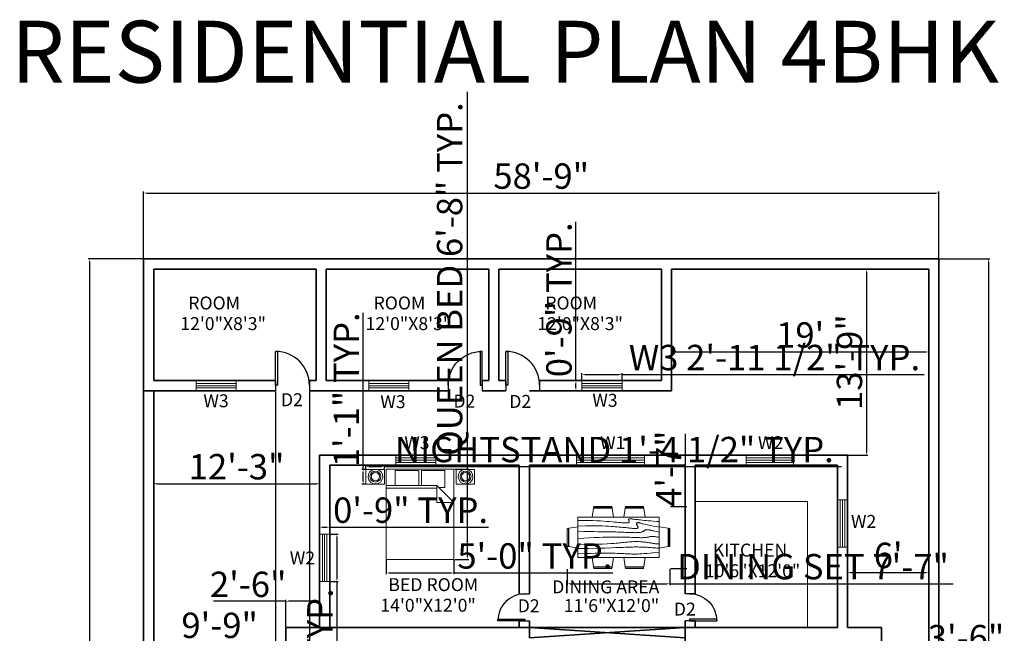
# Model space of a CAD drawing. Units: inches. Extents: x 164 to 1038, y 98 to 1358.
# Tile 4 of 4: x 164 to 1037, y 814 to 1358. Entities that reach past the tile are written whole.
import ezdxf

# ---------------------------------------------------------------- set-up
doc = ezdxf.new("R2010")
doc.units = ezdxf.units.IN
for name, color, linetype, lineweight in [('A-ANNO-DIMS', 7, 'Continuous', 18), ('A-ANNO-TEXT', 3, 'Continuous', 18), ('A-ANNO-TITL', 7, 'Continuous', 35), ('A-AREA-IDEN', 3, 'Continuous', 18), ('A-FLOR-FIXT', 2, 'Continuous', 18), ('C-SITE-WALL', 7, 'Continuous', 35), ('door', 6, 'Continuous', 25), ('furniture', 2, 'Continuous', 18), ('wall', 7, 'Continuous', 35), ('window', 10, 'Continuous', 18)]:
    doc.layers.add(name, color=color, linetype=linetype, lineweight=lineweight)
doc.styles.get("Standard").update_dxf_attribs({"font": 'arial.ttf'})
doc.dimstyles.new('ISO-25', dxfattribs={"dimtxt": 22.5, "dimasz": 2.5, "dimexe": 1.25, "dimexo": 0.625, "dimtad": 1, "dimdec": 0, "dimlunit": 3, "dimtxsty": 'Standard', "dimcen": 2.5, "dimadec": 0, "dimazin": 0, "dimtfac": 1, "dimtdec": 0, "dimtmove": 0, "dimatfit": 3, "dimfxl": 1, "dimarcsym": 0})

# ---------------------------------------------------------------- blocks, each defined once
blk = doc.blocks.new('*U3')
for p, q in [((0, 0), (0, -5)), ((30, 0), (30, -5))]:
    blk.add_line(p, q)
blk.add_lwpolyline([(0, 0), (0, 30), (1.75, 30), (1.75, 0)], close=True)
blk.add_arc((0, 0), 30, 0, 90)
blk = doc.blocks.new('Dining Set - 36 x 72 in.')
for p, q in [((-22, 27.5), (-22.1562, 26.50042)), ((-5.8416, 26.5), (-22.1534, 26.5)), ((-22, 27.5), (-6, 27.5)), ((-5.8437, 26.49966), (-6, 27.5)), ((6, 27.5), (5.8438, 26.50042)), ((22.1584, 26.5), (5.8466, 26.5)), ((6, 27.5), (22, 27.5)), ((22.1563, 26.49966), (22, 27.5)), ((36, 18), (-36, 18)), ((-36, 18), (-36, -18)), ((-22.2343, 26.00059), (-23.4847, 17.99762)), ((-22.2304, 26), (-5.7608, 26)), ((-4.5152, 17.99762), (-5.7655, 25.99926)), ((5.7657, 26.00059), (4.5153, 17.99762)), ((5.7696, 26), (22.2392, 26)), ((23.4848, 17.99762), (22.2345, 25.99926)), ((36, -18), (36, 18)), ((-44.0006, 8.23428), (-35.9976, 9.48474)), ((44.0006, 8.23428), (35.9976, 9.48474)), ((-45.5, 8), (-44.5004, 8.15617)), ((-45.5, 8), (-45.5, -8)), ((-44.5, -8.15843), (-44.5, 8.15338)), ((-44, 8.23041), (-44, -8.23915)), ((44, 8.23041), (44, -8.23915)), ((44.5, -8.15843), (44.5, 8.15338)), ((45.5, 8), (44.5005, 8.15617)), ((45.5, 8), (45.5, -8)), ((-44.4997, -8.15631), (-45.5, -8)), ((-35.9976, -9.48476), (-43.9993, -8.2345)), ((35.9976, -9.48476), (43.9993, -8.2345)), ((44.4997, -8.15631), (45.5, -8)), ((-36, -18), (36, -18)), ((-22.2343, -26.0006), (-23.4847, -17.99762)), ((-22.2304, -26), (-5.7608, -26)), ((-4.5152, -17.99762), (-5.7655, -25.99928)), ((5.7657, -26.0006), (4.5153, -17.99762)), ((5.7696, -26), (22.2392, -26)), ((23.4848, -17.99762), (22.2345, -25.99928)), ((-22, -27.5), (-22.1562, -26.50044)), ((-5.8416, -26.5), (-22.1534, -26.5)), ((-22, -27.5), (-6, -27.5)), ((-5.8437, -26.49967), (-6, -27.5)), ((6, -27.5), (5.8438, -26.50044)), ((22.1584, -26.5), (5.8466, -26.5)), ((6, -27.5), (22, -27.5)), ((22.1563, -26.49967), (22, -27.5))]:
    blk.add_line(p, q)
for points in [[(-36, 15), (-31.1772, 14.97754), (-26.8079, 14.91406), (-22.8538, 14.81543), (-19.276, 14.6875), (-16.0362, 14.53613), (-13.0957, 14.36718), (-10.4159, 14.18652), (-7.9583, 14), (-5.6904, 13.81315), (-3.6035, 13.63021), (-1.6954, 13.45508), (0.0365, 13.29166), (1.5945, 13.14388), (2.9811, 13.01562), (4.1988, 12.9108), (5.25, 12.83333), (6.1393, 12.78613), (6.8802, 12.76823), (7.4883, 12.77767), (7.9792, 12.8125), (8.3685, 12.87077), (8.6719, 12.95052), (8.9049, 13.0498), (9.0833, 13.16666), (9.2205, 13.29899), (9.3216, 13.44401), (9.3895, 13.59879), (9.4271, 13.76041), (9.4373, 13.92594), (9.4232, 14.09245), (9.3875, 14.257), (9.3333, 14.41666), (9.2638, 14.56917), (9.1836, 14.71484), (9.0975, 14.85465), (9.0104, 14.98958), (8.9272, 15.1206), (8.8529, 15.2487), (8.7922, 15.37483), (8.75, 15.5), (8.7305, 15.62467), (8.7344, 15.74739), (8.7617, 15.86621), (8.8125, 15.97916), (8.8867, 16.08431), (8.9844, 16.17968), (9.1055, 16.26334), (9.25, 16.33333), (9.4189, 16.38802), (9.6172, 16.42708), (9.8506, 16.45052), (10.125, 16.45833), (10.4463, 16.45052), (10.8203, 16.42708), (11.2529, 16.38802), (11.75, 16.33333), (12.3184, 16.26318), (12.9694, 16.17838), (13.7151, 16.07991), (14.5677, 15.96875), (15.5395, 15.84586), (16.6426, 15.71224), (17.8893, 15.56884), (19.2917, 15.41666), (20.859, 15.25667), (22.5879, 15.08984), (24.4721, 14.91715), (26.5052, 14.73958), (28.6809, 14.5581), (30.9929, 14.3737), (33.4347, 14.18733), (36, 14)], [(-36, 10), (-28.9766, 10.14274), (-23.1725, 10.20442), (-18.4241, 10.19775), (-14.5677, 10.13541), (-11.4399, 10.03011), (-8.877, 9.89453), (-6.7154, 9.74137), (-4.7917, 9.58333), (-2.9698, 9.43082), (-1.2246, 9.28515), (0.4415, 9.14534), (2.026, 9.01041), (3.5266, 8.87939), (4.9408, 8.7513), (6.266, 8.62516), (7.5, 8.5), (8.6411, 8.37549), (9.6914, 8.2539), (10.6538, 8.13818), (11.5312, 8.03125), (12.3267, 7.93603), (13.043, 7.85547), (13.6831, 7.79248), (14.25, 7.75), (14.7471, 7.7303), (15.1797, 7.73307), (15.5537, 7.75732), (15.875, 7.80208), (16.1494, 7.86637), (16.3828, 7.94922), (16.5811, 8.04964), (16.75, 8.16666), (16.8944, 8.29915), (17.0143, 8.44531), (17.1089, 8.60319), (17.1771, 8.77083), (17.218, 8.94629), (17.2305, 9.1276), (17.2137, 9.31282), (17.1667, 9.5), (17.0895, 9.6875), (16.987, 9.875), (16.8649, 10.0625), (16.7292, 10.25), (16.5856, 10.4375), (16.4401, 10.625), (16.2985, 10.8125), (16.1667, 11), (16.05, 11.18733), (15.9518, 11.3737), (15.8752, 11.5581), (15.8229, 11.73958), (15.798, 11.91715), (15.8034, 12.08984), (15.842, 12.25667), (15.9167, 12.41666), (16.0295, 12.56836), (16.1784, 12.70833), (16.3605, 12.83268), (16.5729, 12.9375), (16.8127, 13.01888), (17.0768, 13.07291), (17.3625, 13.0957), (17.6667, 13.08333), (17.9894, 13.03312), (18.3418, 12.94726), (18.7382, 12.82918), (19.1927, 12.68229), (19.7195, 12.51001), (20.3327, 12.31575), (21.0465, 12.10294), (21.875, 11.875), (22.8357, 11.63354), (23.959, 11.37304), (25.2786, 11.08618), (26.8282, 10.76562), (28.6414, 10.40405), (30.752, 9.99414), (33.1936, 9.52856), (36, 9)], [(-36, 5.5), (-30.7157, 5.3348), (-26.069, 5.20963), (-21.9946, 5.11767), (-18.4271, 5.05208), (-15.3009, 5.00602), (-12.5508, 4.97265), (-10.1112, 4.94515), (-7.9167, 4.91666), (-5.909, 4.88167), (-4.0586, 4.83984), (-2.3429, 4.79215), (-0.7396, 4.73958), (0.7739, 4.6831), (2.22, 4.6237), (3.6213, 4.56233), (5, 4.5), (6.373, 4.43782), (7.7344, 4.3776), (9.0723, 4.32129), (10.375, 4.27083), (11.6309, 4.22819), (12.8281, 4.19531), (13.9551, 4.17415), (15, 4.16666), (15.954, 4.17448), (16.819, 4.19791), (17.6001, 4.23698), (18.3021, 4.29166), (18.9299, 4.36198), (19.4883, 4.44791), (19.9823, 4.54948), (20.4167, 4.66666), (20.7969, 4.79899), (21.1302, 4.94401), (21.4245, 5.09879), (21.6875, 5.26041), (21.9271, 5.42594), (22.1511, 5.59245), (22.3672, 5.757), (22.5834, 5.91666), (22.8065, 6.06868), (23.0404, 6.21093), (23.2879, 6.34147), (23.5521, 6.45833), (23.8358, 6.55957), (24.142, 6.64323), (24.4735, 6.70735), (24.8334, 6.75), (25.2235, 6.76969), (25.642, 6.76692), (26.0858, 6.74267), (26.5521, 6.69791), (27.0379, 6.63362), (27.5404, 6.55078), (28.0565, 6.45036), (28.5834, 6.33333), (29.1242, 6.19987), (29.7071, 6.04687), (30.3661, 5.87044), (31.1354, 5.66666), (32.0493, 5.43164), (33.142, 5.16146), (34.4475, 4.85221), (36, 4.5)], [(-36, -1), (-30.7915, -0.6591), (-26.0195, -0.38216), (-21.6519, -0.16284), (-17.6563, 0.00521), (-14.0005, 0.12833), (-10.6523, 0.21289), (-7.5796, 0.26522), (-4.75, 0.29166), (-2.134, 0.29793), (0.2878, 0.28711), (2.5317, 0.26163), (4.6146, 0.22396), (6.5529, 0.17651), (8.3633, 0.12174), (10.0623, 0.06209), (11.6667, 0), (13.1899, -0.06201), (14.6341, -0.1211), (15.9982, -0.17432), (17.2813, -0.21875), (18.4823, -0.25147), (19.6003, -0.26953), (20.6343, -0.27002), (21.5834, -0.25), (22.4481, -0.20768), (23.2357, -0.14584), (23.9549, -0.06836), (24.6146, 0.02083), (25.2235, 0.11784), (25.7904, 0.21875), (26.3241, 0.31966), (26.8334, 0.41666), (27.3265, 0.50618), (27.8099, 0.58593), (28.2894, 0.65397), (28.7709, 0.70833), (29.2601, 0.74707), (29.763, 0.76823), (30.2855, 0.76985), (30.8334, 0.75), (31.4088, 0.70784), (31.9994, 0.64713), (32.589, 0.57275), (33.1615, 0.48958), (33.7008, 0.4025), (34.1908, 0.3164), (34.6153, 0.23616), (34.9584, 0.16666), (35.2099, 0.11165), (35.3848, 0.07031), (35.504, 0.04069), (35.5886, 0.02083), (35.6594, 0.00879), (35.7377, 0.0026), (35.8442, 0.00032), (36, 0)], [(-36, -6.5), (-27.1843, -6.31267), (-20.084, -6.1263), (-14.469, -5.9419), (-10.1094, -5.76042), (-6.7752, -5.58285), (-4.2363, -5.41016), (-2.2629, -5.24333), (-0.625, -5.08334), (0.8708, -4.93099), (2.2715, -4.78646), (3.5872, -4.64974), (4.8281, -4.52084), (6.0046, -4.39974), (7.127, -4.28646), (8.2053, -4.18099), (9.25, -4.08334), (10.2705, -3.99382), (11.2734, -3.91407), (12.2647, -3.84603), (13.25, -3.79167), (14.2354, -3.75293), (15.2266, -3.73177), (16.2295, -3.73015), (17.25, -3.75), (18.2912, -3.79248), (19.3451, -3.85547), (20.4009, -3.93604), (21.4479, -4.03125), (22.4754, -4.13819), (23.4727, -4.25391), (24.4289, -4.37549), (25.3334, -4.5), (26.1785, -4.62492), (26.9694, -4.74935), (27.7145, -4.87281), (28.4219, -4.99479), (29.1, -5.11483), (29.7572, -5.23242), (30.4016, -5.34709), (31.0417, -5.45834), (31.6837, -5.56437), (32.3262, -5.65821), (32.9658, -5.73153), (33.599, -5.77604), (34.2224, -5.78345), (34.8327, -5.74545), (35.4264, -5.65373), (36, -5.5)], [(-36, -10), (-26.4022, -9.81299), (-18.4675, -9.62891), (-11.9839, -9.45069), (-6.7396, -9.28125), (-2.5226, -9.12354), (0.8789, -8.98047), (3.6769, -8.85498), (6.0833, -8.75), (8.2767, -8.66765), (10.3021, -8.60677), (12.1712, -8.56543), (13.8958, -8.54167), (15.4876, -8.53353), (16.9583, -8.53907), (18.3197, -8.55632), (19.5834, -8.58334), (20.7616, -8.61841), (21.8685, -8.66081), (22.9188, -8.71004), (23.9271, -8.76563), (24.9081, -8.82707), (25.8763, -8.89388), (26.8465, -8.96558), (27.8334, -9.04167), (28.8474, -9.12118), (29.8828, -9.20117), (30.93, -9.27824), (31.9792, -9.34896), (33.0205, -9.40991), (34.0443, -9.45768), (35.0407, -9.48885), (36, -9.5)], [(-36, -14.5), (-30.0881, -14.33513), (-25.0332, -14.21224), (-20.7312, -14.12647), (-17.0781, -14.07292), (-13.97, -14.04671), (-11.3027, -14.04297), (-8.9724, -14.05681), (-6.875, -14.08334), (-4.9224, -14.11833), (-3.0905, -14.16016), (-1.3709, -14.20785), (0.2448, -14.26042), (1.7647, -14.3169), (3.1973, -14.3763), (4.5507, -14.43767), (5.8333, -14.5), (7.0554, -14.5621), (8.235, -14.62175), (9.3922, -14.67652), (10.5469, -14.72396), (11.7192, -14.76164), (12.929, -14.78711), (14.1965, -14.79794), (15.5417, -14.79167), (16.9933, -14.76424), (18.6152, -14.70508), (20.4804, -14.60197), (22.6615, -14.44271), (25.2312, -14.21509), (28.2624, -13.9069), (31.8277, -13.50594), (36, -13)]]:
    blk.add_lwpolyline(points)
blk = doc.blocks.new('Bed - Queen')
for p, q in [((0, -80.00003), (0, 0)), ((0, 0), (59.99999, 0)), ((59.99999, 0), (59.99999, -80.00003)), ((7.99999, -1.2), (28.79998, -1.2)), ((7.99999, -14.4), (7.99999, -1.2)), ((28.79998, -1.2), (28.79998, -14.4)), ((31.19999, -1.2), (51.99999, -1.2)), ((31.19999, -14.4), (31.19999, -1.2)), ((51.99999, -1.2), (51.99999, -16.4)), ((0, -14.4), (44.8, -14.4)), ((44.8, -16.8), (0, -16.8)), ((59.99999, -29.6), (44.8, -14.4)), ((44.8, -14.4), (44.8, -29.6)), ((51.99999, -16.4), (46.79936, -16.4)), ((44.8, -29.6), (59.99999, -29.6)), ((59.99999, -80.00003), (0, -80.00003))]:
    blk.add_line(p, q)
blk = doc.blocks.new('*D17')
at = {"layer": 'A-ANNO-DIMS', "color": 0, "lineweight": -2, "transparency": 16777216}
for p, q in [((274.07, 1146.49), (274.07, 1205.54)), ((276.57, 1204.29), (976.57, 1204.29)), ((979.07, 1146.49), (979.07, 1205.54))]:
    blk.add_line(p, q, dxfattribs=at)
at = {"layer": 'A-ANNO-DIMS', "color": 0, "transparency": 16777216}
for points in [[(276.57, 1204.71), (276.57, 1203.88), (274.07, 1204.29)], [(976.57, 1204.71), (976.57, 1203.88), (979.07, 1204.29)]]:
    blk.add_solid(points, dxfattribs=at)
at = {"layer": 'Defpoints', "color": 0, "transparency": 16777216}
for p in [(979.07, 1204.29), (274.07, 1145.87), (979.07, 1145.87)]:
    blk.add_point(p, dxfattribs=at)
at = {"layer": 'A-ANNO-DIMS', "color": 0, "transparency": 16777216, "insert": (626.57, 1216.41), "char_height": 22.5, "attachment_point": 5}
blk.add_mtext('58\'-9"', dxfattribs=at)
blk = doc.blocks.new('*D19')
at = {"layer": 'A-ANNO-DIMS', "color": 0, "lineweight": -2, "transparency": 16777216}
for p, q in [((979.69, 1145.87), (1024.11, 1145.87)), ((1022.86, 1143.37), (1022.86, 212.37)), ((979.69, 209.87), (1024.11, 209.87))]:
    blk.add_line(p, q, dxfattribs=at)
at = {"layer": 'A-ANNO-DIMS', "color": 0, "transparency": 16777216}
for points in [[(1022.44, 1143.37), (1023.28, 1143.37), (1022.86, 1145.87)], [(1022.44, 212.37), (1023.28, 212.37), (1022.86, 209.87)]]:
    blk.add_solid(points, dxfattribs=at)
at = {"layer": 'Defpoints', "color": 0, "transparency": 16777216}
for p in [(979.07, 1145.87), (979.07, 209.87), (1022.86, 209.87)]:
    blk.add_point(p, dxfattribs=at)
at = {"layer": 'A-ANNO-DIMS', "color": 0, "transparency": 16777216, "insert": (1010.75, 677.87), "char_height": 22.5, "attachment_point": 5, "rotation": 90}
blk.add_mtext("78'", dxfattribs=at)
blk = doc.blocks.new('*D20')
at = {"layer": 'A-ANNO-DIMS', "color": 0, "lineweight": -2, "transparency": 16777216}
for p, q in [((273.44, 1145.87), (224.94, 1145.87)), ((226.19, 1143.37), (226.19, 212.37)), ((273.44, 209.87), (224.94, 209.87))]:
    blk.add_line(p, q, dxfattribs=at)
at = {"layer": 'A-ANNO-DIMS', "color": 0, "transparency": 16777216}
for points in [[(225.78, 1143.37), (226.61, 1143.37), (226.19, 1145.87)], [(225.78, 212.37), (226.61, 212.37), (226.19, 209.87)]]:
    blk.add_solid(points, dxfattribs=at)
at = {"layer": 'Defpoints', "color": 0, "transparency": 16777216}
for p in [(274.07, 1145.87), (226.19, 209.87), (274.07, 209.87)]:
    blk.add_point(p, dxfattribs=at)
at = {"layer": 'A-ANNO-DIMS', "color": 0, "transparency": 16777216, "insert": (214.08, 677.87), "char_height": 22.5, "attachment_point": 5, "rotation": 90}
blk.add_mtext("78'", dxfattribs=at)
blk = doc.blocks.new('*D21')
at = {"layer": 'A-ANNO-DIMS', "color": 0, "lineweight": -2, "transparency": 16777216}
for p, q in [((742.07, 1029.49), (742.07, 1064.58)), ((744.57, 1063.33), (967.57, 1063.33)), ((970.07, 1029.49), (970.07, 1064.58))]:
    blk.add_line(p, q, dxfattribs=at)
at = {"layer": 'A-ANNO-DIMS', "color": 0, "transparency": 16777216}
for points in [[(744.57, 1063.75), (744.57, 1062.92), (742.07, 1063.33)], [(967.57, 1063.75), (967.57, 1062.92), (970.07, 1063.33)]]:
    blk.add_solid(points, dxfattribs=at)
at = {"layer": 'Defpoints', "color": 0, "transparency": 16777216}
for p in [(970.07, 1063.33), (742.07, 1028.87), (970.07, 1028.87)]:
    blk.add_point(p, dxfattribs=at)
at = {"layer": 'A-ANNO-DIMS', "color": 0, "transparency": 16777216, "insert": (856.07, 1075.45), "char_height": 22.5, "attachment_point": 5}
blk.add_mtext("19'", dxfattribs=at)
blk = doc.blocks.new('*D22')
at = {"layer": 'A-ANNO-DIMS', "color": 0, "lineweight": -2, "transparency": 16777216}
for p, q in [((850.76, 1136.87), (916.03, 1136.87)), ((914.78, 1134.37), (914.78, 974.37)), ((850.76, 971.87), (916.03, 971.87))]:
    blk.add_line(p, q, dxfattribs=at)
at = {"layer": 'A-ANNO-DIMS', "color": 0, "transparency": 16777216}
for points in [[(914.36, 1134.37), (915.19, 1134.37), (914.78, 1136.87)], [(914.36, 974.37), (915.19, 974.37), (914.78, 971.87)]]:
    blk.add_solid(points, dxfattribs=at)
at = {"layer": 'Defpoints', "color": 0, "transparency": 16777216}
for p in [(850.14, 1136.87), (850.14, 971.87), (914.78, 971.87)]:
    blk.add_point(p, dxfattribs=at)
at = {"layer": 'A-ANNO-DIMS', "color": 0, "transparency": 16777216, "insert": (902.65, 1054.37), "char_height": 22.5, "attachment_point": 5, "rotation": 90}
blk.add_mtext('13\'-9"', dxfattribs=at)
blk = doc.blocks.new('*D23')
at = {"layer": 'A-ANNO-DIMS', "color": 0, "lineweight": -2, "transparency": 16777216}
for p, q in [((283.07, 908.78), (283.07, 947.73)), ((285.57, 946.48), (427.57, 946.48)), ((430.07, 908.78), (430.07, 947.73))]:
    blk.add_line(p, q, dxfattribs=at)
at = {"layer": 'A-ANNO-DIMS', "color": 0, "transparency": 16777216}
for points in [[(285.57, 946.9), (285.57, 946.06), (283.07, 946.48)], [(427.57, 946.9), (427.57, 946.06), (430.07, 946.48)]]:
    blk.add_solid(points, dxfattribs=at)
at = {"layer": 'Defpoints', "color": 0, "transparency": 16777216}
for p in [(430.07, 946.48), (283.07, 908.16), (430.07, 908.16)]:
    blk.add_point(p, dxfattribs=at)
at = {"layer": 'A-ANNO-DIMS', "color": 0, "transparency": 16777216, "insert": (356.57, 958.6), "char_height": 22.5, "attachment_point": 5}
blk.add_mtext('12\'-3"', dxfattribs=at)
blk = doc.blocks.new('*D24')
at = {"layer": 'A-ANNO-DIMS', "color": 0, "lineweight": -2, "transparency": 16777216}
for p, q in [((283.07, 795.15), (283.07, 807.04)), ((285.57, 805.79), (397.57, 805.79)), ((400.07, 795.15), (400.07, 807.04))]:
    blk.add_line(p, q, dxfattribs=at)
at = {"layer": 'A-ANNO-DIMS', "color": 0, "transparency": 16777216}
for points in [[(285.57, 806.21), (285.57, 805.37), (283.07, 805.79)], [(397.57, 806.21), (397.57, 805.37), (400.07, 805.79)]]:
    blk.add_solid(points, dxfattribs=at)
at = {"layer": 'Defpoints', "color": 0, "transparency": 16777216}
for p in [(400.07, 805.79), (283.07, 794.52), (400.07, 794.52)]:
    blk.add_point(p, dxfattribs=at)
at = {"layer": 'A-ANNO-DIMS', "color": 0, "transparency": 16777216, "insert": (341.57, 817.9), "char_height": 22.5, "attachment_point": 5}
blk.add_mtext('9\'-9"', dxfattribs=at)
blk = doc.blocks.new('*D27')
at = {"layer": 'A-ANNO-DIMS', "color": 0, "lineweight": -2, "transparency": 16777216}
for p, q in [((898.07, 871.04), (898.07, 866.59)), ((900.57, 867.84), (967.57, 867.84)), ((970.07, 871.04), (970.07, 866.59))]:
    blk.add_line(p, q, dxfattribs=at)
at = {"layer": 'A-ANNO-DIMS', "color": 0, "transparency": 16777216}
for points in [[(900.57, 868.25), (900.57, 867.42), (898.07, 867.84)], [(967.57, 868.25), (967.57, 867.42), (970.07, 867.84)]]:
    blk.add_solid(points, dxfattribs=at)
at = {"layer": 'Defpoints', "color": 0, "transparency": 16777216}
for p in [(898.07, 871.66), (970.07, 871.66), (970.07, 867.84)]:
    blk.add_point(p, dxfattribs=at)
at = {"layer": 'A-ANNO-DIMS', "color": 0, "transparency": 16777216, "insert": (934.07, 879.95), "char_height": 22.5, "attachment_point": 5}
blk.add_mtext("6'", dxfattribs=at)
blk = doc.blocks.new('*D28')
at = {"layer": 'A-ANNO-DIMS', "color": 0, "lineweight": -2, "transparency": 16777216}
for p, q in [((928.07, 772.18), (928.07, 796.13)), ((930.57, 794.88), (967.57, 794.88)), ((970.07, 772.18), (970.07, 796.13)), ((970.07, 794.88), (1033.61, 794.88))]:
    blk.add_line(p, q, dxfattribs=at)
at = {"layer": 'A-ANNO-DIMS', "color": 0, "transparency": 16777216}
for points in [[(930.57, 795.3), (930.57, 794.46), (928.07, 794.88)], [(967.57, 795.3), (967.57, 794.46), (970.07, 794.88)]]:
    blk.add_solid(points, dxfattribs=at)
at = {"layer": 'Defpoints', "color": 0, "transparency": 16777216}
for p in [(970.07, 794.88), (928.07, 771.56), (970.07, 771.56)]:
    blk.add_point(p, dxfattribs=at)
at = {"layer": 'A-ANNO-DIMS', "color": 0, "transparency": 16777216, "insert": (1003.09, 807), "char_height": 22.5, "attachment_point": 5}
blk.add_mtext('3\'-6"', dxfattribs=at)
blk = doc.blocks.new('*D29')
at = {"layer": 'A-ANNO-DIMS', "color": 0, "lineweight": -2, "transparency": 16777216}
for p, q in [((400.07, 842.17), (336.12, 842.17)), ((400.07, 819.49), (400.07, 843.42)), ((427.57, 842.17), (402.57, 842.17)), ((430.07, 819.49), (430.07, 843.42))]:
    blk.add_line(p, q, dxfattribs=at)
at = {"layer": 'A-ANNO-DIMS', "color": 0, "transparency": 16777216}
for points in [[(402.57, 842.59), (402.57, 841.75), (400.07, 842.17)], [(427.57, 842.59), (427.57, 841.75), (430.07, 842.17)]]:
    blk.add_solid(points, dxfattribs=at)
at = {"layer": 'Defpoints', "color": 0, "transparency": 16777216}
for p in [(400.07, 842.17), (400.07, 818.87), (430.07, 818.87)]:
    blk.add_point(p, dxfattribs=at)
at = {"layer": 'A-ANNO-DIMS', "color": 0, "transparency": 16777216, "insert": (366.84, 854.28), "char_height": 22.5, "attachment_point": 5}
blk.add_mtext('2\'-6"', dxfattribs=at)
blk = doc.blocks.new('WINDOW-W3')
for p, q in [((0, 9), (0, 0)), ((0, 9), (0, 0)), ((35.59, 9), (35.59, 0)), ((35.59, 9), (35.59, 0)), ((0, 6.5), (35.59, 6.5)), ((0, 6.5), (35.59, 6.5)), ((0, 4.5), (35.59, 4.5)), ((0, 4.5), (35.59, 4.5)), ((0, 2.5), (35.59, 2.5)), ((0, 2.5), (35.59, 2.5))]:
    blk.add_line(p, q)
blk = doc.blocks.new('WINDOW-W1')
for p, q in [((0, 9), (0, 0)), ((60.11, 9), (60.11, 0)), ((0, 6.5), (60.11, 6.5)), ((0, 4.5), (60.11, 4.5)), ((0, 2.5), (60.11, 2.5))]:
    blk.add_line(p, q)
blk = doc.blocks.new('WINDOW-W2')
for p, q in [((0, 9), (0, 0)), ((42.02, 9), (42.02, 0)), ((0, 6.5), (42.02, 6.5)), ((0, 4.5), (42.02, 4.5)), ((0, 2.5), (42.02, 2.5))]:
    blk.add_line(p, q)
blk = doc.blocks.new('BEDSIDE-TABLE')
blk.add_lwpolyline([(0, 13.01), (16.36, 13.01), (16.36, 0), (0, 0)], close=True)
for radius in [4.87, 3.63]:
    blk.add_circle((8.46, 6.65), radius)
blk.add_arc((8.46, 6.65), 6.51, 102.02927, 77.97073)
blk.add_arc((8.46, 6.65), 6.51, 102.02927, 77.97073)
blk = doc.blocks.new('*D36')
at = {"layer": 'A-ANNO-DIMS', "color": 0, "lineweight": -2, "transparency": 16777216}
for p, q in [((439.69, 901.66), (446.62, 901.66)), ((445.37, 899.16), (445.37, 862.14)), ((439.69, 859.64), (446.62, 859.64)), ((445.37, 859.64), (445.37, 661.94))]:
    blk.add_line(p, q, dxfattribs=at)
at = {"layer": 'A-ANNO-DIMS', "color": 0, "transparency": 16777216}
for points in [[(444.95, 899.16), (445.79, 899.16), (445.37, 901.66)], [(444.95, 862.14), (445.79, 862.14), (445.37, 859.64)]]:
    blk.add_solid(points, dxfattribs=at)
at = {"layer": 'Defpoints', "color": 0, "transparency": 16777216}
for p in [(439.07, 901.66), (439.07, 859.64), (445.37, 859.64)]:
    blk.add_point(p, dxfattribs=at)
at = {"layer": 'A-ANNO-DIMS', "color": 0, "transparency": 16777216, "insert": (433.25, 759.54), "char_height": 22.5, "attachment_point": 5, "rotation": 90}
blk.add_mtext('W2 3\'-6" TYP.', dxfattribs=at)
blk = doc.blocks.new('*D37')
at = {"layer": 'A-ANNO-DIMS', "color": 0, "lineweight": -2, "transparency": 16777216}
for p, q in [((430.07, 902.28), (430.07, 909.21)), ((432.57, 907.96), (436.57, 907.96)), ((439.07, 902.28), (439.07, 909.21)), ((439.07, 907.96), (579.97, 907.96))]:
    blk.add_line(p, q, dxfattribs=at)
at = {"layer": 'A-ANNO-DIMS', "color": 0, "transparency": 16777216}
for points in [[(432.57, 908.38), (432.57, 907.54), (430.07, 907.96)], [(436.57, 908.38), (436.57, 907.54), (439.07, 907.96)]]:
    blk.add_solid(points, dxfattribs=at)
at = {"layer": 'Defpoints', "color": 0, "transparency": 16777216}
for p in [(439.07, 907.96), (430.07, 901.66), (439.07, 901.66)]:
    blk.add_point(p, dxfattribs=at)
at = {"layer": 'A-ANNO-DIMS', "color": 0, "transparency": 16777216, "insert": (510.77, 920.07), "char_height": 22.5, "attachment_point": 5}
blk.add_mtext('0\'-9" TYP.', dxfattribs=at)
blk = doc.blocks.new('*D38')
at = {"layer": 'A-ANNO-DIMS', "color": 0, "lineweight": -2, "transparency": 16777216}
for p, q in [((662.65, 1038.49), (662.65, 1044.45)), ((665.15, 1043.2), (695.74, 1043.2)), ((698.24, 1038.49), (698.24, 1044.45)), ((698.24, 1043.2), (965.85, 1043.2))]:
    blk.add_line(p, q, dxfattribs=at)
at = {"layer": 'A-ANNO-DIMS', "color": 0, "transparency": 16777216}
for points in [[(665.15, 1043.62), (665.15, 1042.79), (662.65, 1043.2)], [(695.74, 1043.62), (695.74, 1042.79), (698.24, 1043.2)]]:
    blk.add_solid(points, dxfattribs=at)
at = {"layer": 'Defpoints', "color": 0, "transparency": 16777216}
for p in [(698.24, 1043.2), (662.65, 1037.87), (698.24, 1037.87)]:
    blk.add_point(p, dxfattribs=at)
at = {"layer": 'A-ANNO-DIMS', "color": 0, "transparency": 16777216, "insert": (833.29, 1055.47), "char_height": 22.5, "attachment_point": 5}
blk.add_mtext('W3 2\'-11 1/2" TYP.', dxfattribs=at)
blk = doc.blocks.new('*D39')
at = {"layer": 'A-ANNO-DIMS', "color": 0, "lineweight": -2, "transparency": 16777216}
for p, q in [((657.31, 1037.87), (657.31, 1178.76)), ((662.02, 1037.87), (656.06, 1037.87)), ((657.31, 1031.37), (657.31, 1035.37)), ((662.02, 1028.87), (656.06, 1028.87))]:
    blk.add_line(p, q, dxfattribs=at)
at = {"layer": 'A-ANNO-DIMS', "color": 0, "transparency": 16777216}
for points in [[(656.89, 1035.37), (657.73, 1035.37), (657.31, 1037.87)], [(656.89, 1031.37), (657.73, 1031.37), (657.31, 1028.87)]]:
    blk.add_solid(points, dxfattribs=at)
at = {"layer": 'Defpoints', "color": 0, "transparency": 16777216}
for p in [(657.31, 1037.87), (662.65, 1037.87), (662.65, 1028.87)]:
    blk.add_point(p, dxfattribs=at)
at = {"layer": 'A-ANNO-DIMS', "color": 0, "transparency": 16777216, "insert": (645.2, 1109.57), "char_height": 22.5, "attachment_point": 5, "rotation": 90}
blk.add_mtext('0\'-9" TYP.', dxfattribs=at)
blk = doc.blocks.new('*D40')
at = {"layer": 'A-ANNO-DIMS', "color": 0, "lineweight": -2, "transparency": 16777216}
for p, q in [((561.22, 959.36), (561.22, 1294.09)), ((549.84, 959.36), (562.47, 959.36)), ((561.22, 881.86), (561.22, 956.86)), ((549.84, 879.36), (562.47, 879.36))]:
    blk.add_line(p, q, dxfattribs=at)
at = {"layer": 'A-ANNO-DIMS', "color": 0, "transparency": 16777216}
for points in [[(560.8, 956.86), (561.63, 956.86), (561.22, 959.36)], [(560.8, 881.86), (561.63, 881.86), (561.22, 879.36)]]:
    blk.add_solid(points, dxfattribs=at)
at = {"layer": 'Defpoints', "color": 0, "transparency": 16777216}
for p in [(549.22, 959.36), (561.22, 959.36), (549.22, 879.36)]:
    blk.add_point(p, dxfattribs=at)
at = {"layer": 'A-ANNO-DIMS', "color": 0, "transparency": 16777216, "insert": (548.27, 1127.98), "char_height": 22.5, "attachment_point": 5, "rotation": 90}
blk.add_mtext('QUEEN BED 6\'-8" TYP.', dxfattribs=at)
blk = doc.blocks.new('*D41')
at = {"layer": 'A-ANNO-DIMS', "color": 0, "lineweight": -2, "transparency": 16777216}
for p, q in [((489.22, 878.74), (489.22, 866.11)), ((549.22, 878.74), (549.22, 866.11)), ((491.72, 867.36), (546.72, 867.36)), ((549.22, 867.36), (690.11, 867.36))]:
    blk.add_line(p, q, dxfattribs=at)
at = {"layer": 'A-ANNO-DIMS', "color": 0, "transparency": 16777216}
for points in [[(491.72, 867.78), (491.72, 866.95), (489.22, 867.36)], [(546.72, 867.78), (546.72, 866.95), (549.22, 867.36)]]:
    blk.add_solid(points, dxfattribs=at)
at = {"layer": 'Defpoints', "color": 0, "transparency": 16777216}
for p in [(489.22, 879.36), (549.22, 879.36), (549.22, 867.36)]:
    blk.add_point(p, dxfattribs=at)
at = {"layer": 'A-ANNO-DIMS', "color": 0, "transparency": 16777216, "insert": (620.92, 879.48), "char_height": 22.5, "attachment_point": 5}
blk.add_mtext('5\'-0" TYP.', dxfattribs=at)
blk = doc.blocks.new('*D42')
at = {"layer": 'A-ANNO-DIMS', "color": 0, "lineweight": -2, "transparency": 16777216}
for p, q in [((471.16, 959.77), (471.16, 962.84)), ((473.66, 961.59), (485.01, 961.59)), ((487.51, 959.77), (487.51, 962.84)), ((487.51, 961.59), (892.8, 961.59))]:
    blk.add_line(p, q, dxfattribs=at)
at = {"layer": 'A-ANNO-DIMS', "color": 0, "transparency": 16777216}
for points in [[(473.66, 962.01), (473.66, 961.18), (471.16, 961.59)], [(485.01, 962.01), (485.01, 961.18), (487.51, 961.59)]]:
    blk.add_solid(points, dxfattribs=at)
at = {"layer": 'Defpoints', "color": 0, "transparency": 16777216}
for p in [(487.51, 961.59), (471.16, 959.14), (487.51, 959.14)]:
    blk.add_point(p, dxfattribs=at)
at = {"layer": 'A-ANNO-DIMS', "color": 0, "transparency": 16777216, "insert": (691.4, 973.85), "char_height": 22.5, "attachment_point": 5}
blk.add_mtext('NIGHTSTAND 1\'-4 1/2" TYP.', dxfattribs=at)
blk = doc.blocks.new('*D43')
at = {"layer": 'A-ANNO-DIMS', "color": 0, "lineweight": -2, "transparency": 16777216}
for p, q in [((468.7, 959.14), (468.7, 1097.92)), ((470.53, 959.14), (467.45, 959.14)), ((468.7, 948.63), (468.7, 956.64)), ((470.53, 946.13), (467.45, 946.13))]:
    blk.add_line(p, q, dxfattribs=at)
at = {"layer": 'A-ANNO-DIMS', "color": 0, "transparency": 16777216}
for points in [[(468.29, 956.64), (469.12, 956.64), (468.7, 959.14)], [(468.29, 948.63), (469.12, 948.63), (468.7, 946.13)]]:
    blk.add_solid(points, dxfattribs=at)
at = {"layer": 'Defpoints', "color": 0, "transparency": 16777216}
for p in [(468.7, 959.14), (471.16, 959.14), (471.16, 946.13)]:
    blk.add_point(p, dxfattribs=at)
at = {"layer": 'A-ANNO-DIMS', "color": 0, "transparency": 16777216, "insert": (456.77, 1029.78), "char_height": 22.5, "attachment_point": 5, "rotation": 90}
blk.add_mtext('1\'-1" TYP.', dxfattribs=at)
blk = doc.blocks.new('*D48')
at = {"layer": 'A-ANNO-DIMS', "color": 0, "lineweight": -2, "transparency": 16777216}
for p, q in [((649.65, 870.75), (649.65, 856.47)), ((740.65, 870.75), (740.65, 856.47)), ((652.15, 857.72), (738.15, 857.72)), ((740.65, 857.72), (991.7, 857.72))]:
    blk.add_line(p, q, dxfattribs=at)
at = {"layer": 'A-ANNO-DIMS', "color": 0, "transparency": 16777216}
for points in [[(652.15, 858.14), (652.15, 857.31), (649.65, 857.72)], [(738.15, 858.14), (738.15, 857.31), (740.65, 857.72)]]:
    blk.add_solid(points, dxfattribs=at)
at = {"layer": 'Defpoints', "color": 0, "transparency": 16777216}
for p in [(649.65, 871.37), (740.65, 871.37), (740.65, 857.72)]:
    blk.add_point(p, dxfattribs=at)
at = {"layer": 'A-ANNO-DIMS', "color": 0, "transparency": 16777216, "insert": (867.42, 869.98), "char_height": 22.5, "attachment_point": 5}
blk.add_mtext('DINING SET 7\'-7"', dxfattribs=at)
blk = doc.blocks.new('*D49')
at = {"layer": 'A-ANNO-DIMS', "color": 0, "lineweight": -2, "transparency": 16777216}
for p, q in [((754.3, 926.37), (754.3, 990.84)), ((741.27, 926.37), (755.55, 926.37)), ((754.3, 873.87), (754.3, 923.87)), ((741.27, 871.37), (755.55, 871.37))]:
    blk.add_line(p, q, dxfattribs=at)
at = {"layer": 'A-ANNO-DIMS', "color": 0, "transparency": 16777216}
for points in [[(753.88, 923.87), (754.72, 923.87), (754.3, 926.37)], [(753.88, 873.87), (754.72, 873.87), (754.3, 871.37)]]:
    blk.add_solid(points, dxfattribs=at)
at = {"layer": 'Defpoints', "color": 0, "transparency": 16777216}
for p in [(740.65, 926.37), (754.3, 926.37), (740.65, 871.37)]:
    blk.add_point(p, dxfattribs=at)
at = {"layer": 'A-ANNO-DIMS', "color": 0, "transparency": 16777216, "insert": (742.42, 959.86), "char_height": 22.5, "attachment_point": 5, "rotation": 90}
blk.add_mtext('4\'-7"', dxfattribs=at)
blk = doc.blocks.new('*D54')
at = {"layer": 'A-ANNO-DIMS', "color": 0, "lineweight": -2, "transparency": 16777216}
for p, q in [((391.07, 1028.24), (391.07, 152.07)), ((421.07, 1028.24), (421.07, 152.07)), ((393.57, 153.32), (418.57, 153.32)), ((421.07, 153.32), (485.01, 153.32))]:
    blk.add_line(p, q, dxfattribs=at)
at = {"layer": 'A-ANNO-DIMS', "color": 0, "transparency": 16777216}
for points in [[(393.57, 153.73), (393.57, 152.9), (391.07, 153.32)], [(418.57, 153.73), (418.57, 152.9), (421.07, 153.32)]]:
    blk.add_solid(points, dxfattribs=at)
at = {"layer": 'Defpoints', "color": 0, "transparency": 16777216}
for p in [(391.07, 1028.87), (421.07, 1028.87), (421.07, 153.32)]:
    blk.add_point(p, dxfattribs=at)
at = {"layer": 'A-ANNO-DIMS', "color": 0, "transparency": 16777216, "insert": (454.29, 165.43), "char_height": 22.5, "attachment_point": 5}
blk.add_mtext('2\'-6"', dxfattribs=at)
blk = doc.blocks.new('*D63')
at = {"layer": 'A-ANNO-DIMS', "color": 0, "lineweight": -2, "transparency": 16777216}
for p, q in [((576.82, 773.71), (574.32, 773.71)), ((579.32, 773.71), (607.44, 773.71)), ((745.52, 773.71), (609.94, 773.71))]:
    blk.add_line(p, q, dxfattribs=at)
at = {"layer": 'A-ANNO-DIMS', "color": 0, "transparency": 16777216}
for points in [[(576.82, 774.13), (576.82, 773.29), (579.32, 773.71)], [(609.94, 774.13), (609.94, 773.29), (607.44, 773.71)]]:
    blk.add_solid(points, dxfattribs=at)
at = {"layer": 'Defpoints', "color": 0, "transparency": 16777216}
for p in [(579.32, 773.71), (607.44, 773.71)]:
    blk.add_point(p, dxfattribs=at)
at = {"layer": 'A-ANNO-DIMS', "color": 0, "transparency": 16777216, "insert": (678.98, 786.45), "char_height": 22.5, "attachment_point": 5, "rotation": 359.99999}
blk.add_mtext('2X ∅2\'-4"', dxfattribs=at)

msp = doc.modelspace()

# ---------------------------------------------------------------- linework, layer by layer
at = {"layer": 'A-FLOR-FIXT'}
for p, q in [((763.07, 930.8), (862.46, 930.8)), ((862.46, 930.8), (862.46, 818.87))]:
    msp.add_line(p, q, dxfattribs=at)
at = {"layer": 'C-SITE-WALL'}
for p, q in [((979.07, 1145.87), (274.07, 1145.87)), ((274.07, 1145.87), (274.07, 209.87)), ((979.07, 1145.87), (979.07, 209.87)), ((970.07, 1136.87), (742.07, 1136.87)), ((970.07, 1136.87), (970.07, 962.49)), ((283.07, 1028.87), (283.07, 662.87)), ((970.07, 962.87), (970.07, 818.87)), ((970.07, 818.87), (970.07, 218.87))]:
    msp.add_line(p, q, dxfattribs=at)
at = {"layer": 'door'}
for p, q in [((391.07, 1037.87), (391.07, 1028.87)), ((421.07, 1037.87), (421.07, 1028.87)), ((544.07, 1037.87), (544.07, 1028.87)), ((574.07, 1037.87), (574.07, 1028.87)), ((595.07, 1037.87), (595.07, 1028.87)), ((625.07, 1037.87), (625.07, 1028.87)), ((607.07, 848.87), (616.07, 848.87)), ((763.07, 848.87), (754.07, 848.87)), ((607.07, 824.87), (616.07, 824.87)), ((763.07, 824.87), (754.07, 824.87))]:
    msp.add_line(p, q, dxfattribs=at)
at = {"layer": 'wall'}
for p, q in [((283.07, 1136.87), (283.07, 1037.87)), ((427.07, 1136.87), (283.07, 1136.87)), ((427.07, 1136.87), (427.07, 1037.87)), ((436.07, 1136.87), (436.07, 1037.87)), ((580.07, 1136.87), (436.07, 1136.87)), ((580.07, 1136.87), (580.07, 1037.87)), ((589.07, 1136.87), (589.07, 1037.87)), ((733.07, 1136.87), (589.07, 1136.87)), ((733.07, 1136.87), (733.07, 1037.87)), ((742.07, 1136.87), (742.07, 1028.87)), ((391.07, 1037.87), (283.07, 1037.87)), ((427.07, 1037.87), (421.07, 1037.87)), ((544.07, 1037.87), (436.07, 1037.87)), ((544.07, 1037.87), (436.07, 1037.87)), ((580.07, 1037.87), (574.07, 1037.87)), ((595.07, 1037.87), (589.07, 1037.87)), ((733.07, 1037.87), (625.07, 1037.87)), ((733.07, 1037.87), (625.07, 1037.87)), ((391.07, 1028.87), (274.07, 1028.87)), ((544.07, 1028.87), (421.07, 1028.87)), ((544.07, 1028.87), (427.07, 1028.87)), ((595.07, 1028.87), (574.07, 1028.87)), ((733.07, 1028.87), (616.07, 1028.87)), ((742.07, 1028.87), (625.07, 1028.87)), ((898.07, 971.87), (430.07, 971.87)), ((430.07, 971.87), (430.07, 818.87)), ((898.07, 971.87), (898.07, 818.87)), ((439.07, 962.87), (439.07, 818.87)), ((607.07, 962.87), (439.07, 962.87)), ((607.07, 962.87), (607.07, 848.87)), ((616.07, 962.87), (616.07, 848.87)), ((754.07, 962.87), (616.07, 962.87)), ((754.07, 962.87), (754.07, 848.87)), ((754.07, 962.87), (754.07, 848.87)), ((889.07, 962.87), (763.07, 962.87)), ((763.07, 962.87), (763.07, 848.87)), ((763.07, 962.87), (763.07, 848.87)), ((889.07, 962.87), (889.07, 818.87)), ((607.07, 824.87), (607.07, 818.87)), ((616.07, 824.87), (616.07, 809.87)), ((754.07, 824.87), (754.07, 818.87)), ((754.07, 824.87), (754.07, 818.87)), ((763.07, 824.87), (763.07, 818.87)), ((763.07, 824.87), (763.07, 818.87)), ((400.07, 818.87), (400.07, 662.87)), ((889.07, 818.87), (400.07, 818.87)), ((616.07, 818.87), (754.07, 809.87)), ((754.07, 818.87), (616.07, 809.87)), ((754.07, 818.87), (754.07, 550.37)), ((928.07, 818.87), (898.07, 818.87)), ((928.07, 818.87), (928.07, 352.37))]:
    msp.add_line(p, q, dxfattribs=at)

# ---------------------------------------------------------------- block references
at = {"layer": 'door'}
for p in [(391.07, 1033.87), (595.07, 1033.87)]:
    msp.add_blockref('*U3', p, dxfattribs=at)
at = {"layer": 'door', "xscale": -1}
msp.add_blockref('*U3', (574.07, 1033.87), dxfattribs=at)
at = {"layer": 'door', "yscale": 0.800000000000003, "zscale": 0.800000000000003}
for p, xscale, rotation in [((612.07, 824.87), 0.800000000000003, 90), ((758.07, 824.87), -0.800000000000003, 270)]:
    msp.add_blockref('*U3', p, dxfattribs=dict(at, xscale=xscale, rotation=rotation))
at = {"layer": 'furniture'}
for name, p in [('BEDSIDE-TABLE', (471.16, 946.13)), ('Bed - Queen', (489.22, 959.36)), ('BEDSIDE-TABLE', (551.04, 946.13)), ('Dining Set - 36 x 72 in.', (695.15, 898.87))]:
    msp.add_blockref(name, p, dxfattribs=at)
at = {"layer": 'window'}
for name, p in [('WINDOW-W3', (320.65, 1028.87)), ('WINDOW-W3', (473.65, 1028.87)), ('WINDOW-W3', (662.65, 1028.87)), ('WINDOW-W3', (497.65, 962.87)), ('WINDOW-W1', (657.87, 962.87)), ('WINDOW-W2', (808.12, 962.87))]:
    msp.add_blockref(name, p, dxfattribs=at)
for p, rotation in [((889.07, 932.31), 270.0000000000007), ((430.07, 901.66), 270.0000000000003)]:
    msp.add_blockref('WINDOW-W2', p, dxfattribs=dict(at, rotation=rotation))

# ---------------------------------------------------------------- texts
at = {"layer": 'A-ANNO-TEXT'}
for s, p in [('W3', (327.14, 1014.24)), ('D2', (395.9, 1015.24)), ('W3', (483.91, 1013.49)), ('D2', (548.74, 1013.97)), ('D2', (598.25, 1013.72)), ('W3', (671.85, 1014.73)), ('W3', (505.18, 977.16)), ('W1', (678.71, 977.13)), ('W2', (818.61, 977.13)), ('W2', (901.11, 907.28)), ('W2', (403.71, 874.88)), ('D2', (605.73, 832.46)), ('D2', (744.1, 829.53))]:
    msp.add_text(s, height=11.466, dxfattribs=at).set_placement(p)
at = {"layer": 'A-ANNO-TITL'}
msp.add_text('RESIDENTIAL PLAN 4BHK', height=54.869, dxfattribs=at).set_placement((156.76, 1302.23))
at = {"layer": 'A-AREA-IDEN'}
for s, height, p in [('ROOM', 11.466, (313.77, 1101.05)), ('ROOM', 11.466, (477.97, 1101.05)), ('ROOM', 11.466, (630.17, 1101.05)), ('12\'0"X8\'3"', 11.466, (306.68, 1082.73)), ('12\'0"X8\'3"', 11.466, (470.89, 1082.73)), ('12\'0"X8\'3"', 11.466, (623.08, 1082.73)), ('KITCHEN', 11.466, (778.66, 881.84)), ('10\'6"X12\'0"', 11.4664, (771.58, 863.52)), ('BED ROOM', 11.466, (491.08, 851.21)), ('DINING AREA', 11.4664, (636.26, 849.2)), ('14\'0"X12\'0"', 11.4664, (483.99, 832.9)), ('11\'6"X12\'0"', 11.4664, (646.5, 832.63))]:
    msp.add_text(s, height=height, dxfattribs=at).set_placement(p)

# ---------------------------------------------------------------- dimensions: what is measured, and where the dimension line sits
at = {"layer": 'A-ANNO-DIMS'}
for base, p1, p2, angle, text, picture, middle in [((561.22, 959.36), (549.22, 879.36), (549.22, 959.36), 90, 'QUEEN BED <> TYP.', '*D40', (548.27, 1127.98)), ((657.31, 1037.87), (662.65, 1028.87), (662.65, 1037.87), 90, '<> TYP.', '*D39', (645.2, 1109.57)), ((468.7, 959.14), (471.16, 946.13), (471.16, 959.14), 90, '<> TYP.', '*D43', (456.77, 1029.78)), ((445.37, 859.64), (439.07, 901.66), (439.07, 859.64), 270, 'W2 <> TYP.', '*D36', (433.25, 759.54))]:
    dim = msp.add_linear_dim(base=base, p1=p1, p2=p2, angle=angle, text=text, dimstyle='ISO-25', override={"dimdec": 1, "dimlfac": 1, "dimrnd": 0, "dimzin": 1, "dimdsep": 46, "dimlunit": 4, "dimfrac": 2}, dxfattribs=at)
    dim.commit()
    dim.dimension.update_dxf_attribs({"geometry": picture, "text_midpoint": middle})
for base, p1, p2, override, picture, middle in [((979.07, 1204.29), (274.07, 1145.87), (979.07, 1145.87), {"dimclrd": 0, "dimclre": 0, "dimclrt": 0}, '*D17', (626.57, 1216.41)), ((970.07, 1063.33), (742.07, 1028.87), (970.07, 1028.87), {"dimclrd": 0, "dimclre": 0, "dimclrt": 0}, '*D21', (856.07, 1075.45)), ((421.07, 153.32), (391.07, 1028.87), (421.07, 1028.87), {"dimdec": 1, "dimlfac": 1, "dimrnd": 0, "dimzin": 1, "dimdsep": 46, "dimlunit": 4, "dimfrac": 2}, '*D54', (454.29, 165.43)), ((430.07, 946.48), (283.07, 908.16), (430.07, 908.16), {"dimclrd": 0, "dimclre": 0, "dimclrt": 0}, '*D23', (356.57, 958.6)), ((970.07, 867.84), (898.07, 871.66), (970.07, 871.66), {"dimclrd": 0, "dimclre": 0, "dimclrt": 0}, '*D27', (934.07, 879.95)), ((400.07, 842.17), (430.07, 818.87), (400.07, 818.87), {"dimclrd": 0, "dimclre": 0, "dimclrt": 0}, '*D29', (366.84, 854.28)), ((400.07, 805.79), (283.07, 794.52), (400.07, 794.52), {"dimclrd": 0, "dimclre": 0, "dimclrt": 0}, '*D24', (341.57, 817.9)), ((970.07, 794.88), (928.07, 771.56), (970.07, 771.56), {"dimclrd": 0, "dimclre": 0, "dimclrt": 0}, '*D28', (1003.09, 807))]:
    dim = msp.add_linear_dim(base=base, p1=p1, p2=p2, dimstyle='ISO-25', override=override, dxfattribs=at)
    dim.commit()
    dim.dimension.update_dxf_attribs({"geometry": picture, "text_midpoint": middle})
for base, p1, p2, override, picture, middle in [((226.19, 209.87), (274.07, 1145.87), (274.07, 209.87), {"dimclrd": 0, "dimclre": 0, "dimclrt": 0}, '*D20', (214.08, 677.87)), ((1022.86, 209.87), (979.07, 1145.87), (979.07, 209.87), {"dimclrd": 0, "dimclre": 0, "dimclrt": 0}, '*D19', (1010.75, 677.87)), ((914.78, 971.87), (850.14, 1136.87), (850.14, 971.87), {"dimclrd": 0, "dimclre": 0, "dimclrt": 0}, '*D22', (902.65, 1054.37)), ((754.3, 926.37), (740.65, 871.37), (740.65, 926.37), {"dimdec": 1, "dimlfac": 1, "dimrnd": 0, "dimzin": 1, "dimdsep": 46, "dimlunit": 4, "dimfrac": 2}, '*D49', (742.42, 959.86))]:
    dim = msp.add_linear_dim(base=base, p1=p1, p2=p2, angle=90, dimstyle='ISO-25', override=override, dxfattribs=at)
    dim.commit()
    dim.dimension.update_dxf_attribs({"geometry": picture, "text_midpoint": middle})
for base, p1, p2, text, picture, middle in [((698.24, 1043.2), (662.65, 1037.87), (698.24, 1037.87), 'W3 <> TYP.', '*D38', (833.29, 1055.47)), ((487.5137, 961.5941), (471.1564, 959.1405), (487.5137, 959.1405), 'NIGHTSTAND <> TYP.', '*D42', (691.4044, 973.8528)), ((439.07, 907.96), (430.07, 901.66), (439.07, 901.66), '<> TYP.', '*D37', (510.77, 920.07)), ((740.65, 857.72), (649.65, 871.37), (740.65, 871.37), 'DINING SET <>', '*D48', (867.42, 869.98)), ((549.22, 867.36), (489.22, 879.36), (549.22, 879.36), '<> TYP.', '*D41', (620.92, 879.48))]:
    dim = msp.add_linear_dim(base=base, p1=p1, p2=p2, text=text, dimstyle='ISO-25', override={"dimdec": 1, "dimlfac": 1, "dimrnd": 0, "dimzin": 1, "dimdsep": 46, "dimlunit": 4, "dimfrac": 2}, dxfattribs=at)
    dim.commit()
    dim.dimension.update_dxf_attribs({"geometry": picture, "text_midpoint": middle})
dim = msp.add_diameter_dim_2p(p1=(579.32, 773.71), p2=(607.44, 773.71), text='2X <>', dimstyle='ISO-25', override={"dimdec": 1, "dimlfac": 1, "dimrnd": 0, "dimzin": 1, "dimdsep": 46, "dimlunit": 4, "dimfrac": 2}, dxfattribs=at)
dim.commit()
dim.dimension.update_dxf_attribs({"geometry": '*D63', "text_midpoint": (678.98, 773.71)})

doc.saveas('drawing.dxf')
